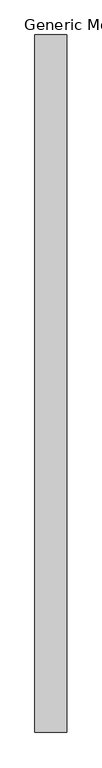
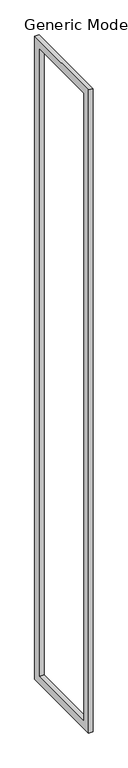
"""IFC4 building model written with IfcOpenShell, lengths in millimetres: proxy geometry, Generic Models 13 : Generic Models 13."""

from ifc_helpers import new_model, si_unit, frame, origin, place, context, project, spatial, polyline, outline, extrude, source, transform, mapped, element, save


def generic_models_13_generic_models_13_61cfa3f2(model_context):
    return source(origin(), model_context, "Body", "SweptSolid", [
        extrude(outline(polyline([(-1125.3142532, 9245.6), (-1125.3142532, 1117.6), (-2242.9142532, 1117.6), (-2242.9142532, 9245.6), (-1125.3142532, 9245.6)]), holes=[polyline([(-1226.9142532, 9144.0), (-2141.3142532, 9144.0), (-2141.3142532, 1219.2), (-1226.9142532, 1219.2), (-1226.9142532, 9144.0)])]), frame((1894.6218735, 0.0, 0.0), z_axis=(1.0, 0.0, 0.0), x_axis=(0.0, 1.0, 0.0)), (0.0, 0.0, 1.0), 50.8),
    ])


if __name__ == "__main__":
    model = new_model("IFC4")
    model_context = context("Model", 3, world=origin())
    ifc_project = project(units=[si_unit("LENGTHUNIT", "METRE", prefix="MILLI")], contexts=[model_context])
    site = spatial("IfcSite", under=ifc_project)
    building = spatial("IfcBuilding", under=site)
    placement = place(None, origin())
    generic_models_13_generic_models_13_shape = generic_models_13_generic_models_13_61cfa3f2(model_context)
    element("IfcBuildingElementProxy", 1, Name="Generic Models 13 : Generic Models 13", ObjectType="Generic Models 13 : Generic Models 13", at=placement, inside=building, context=model_context, shape_type="MappedRepresentation", body=[
        mapped(generic_models_13_generic_models_13_shape, transform((0.0, 0.0, 0.0), x_axis=(1.0, 0.0, 0.0), y_axis=(0.0, 1.0, 0.0), z_axis=(0.0, 0.0, 1.0))),
    ])
    save(model, "model.ifc")
